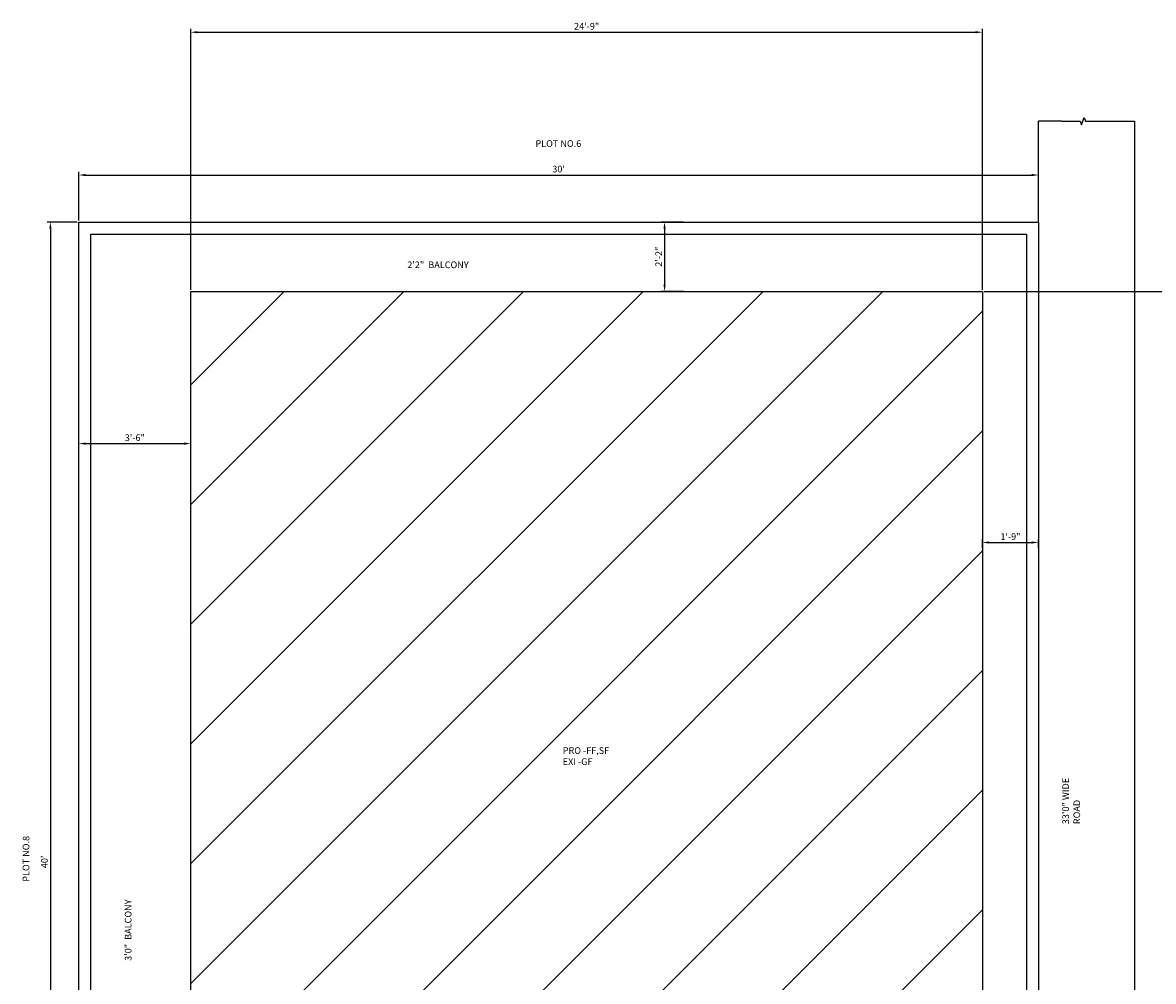
# Model space of a CAD drawing. Units: inches. Extents: x 2020 to 7901, y 1581 to 3943.
# Tile 13 of 17: x 3508 to 3932, y 1955 to 2315. Entities that reach past the tile are written whole.
import ezdxf

# ---------------------------------------------------------------- set-up
doc = ezdxf.new("R2010")
doc.units = ezdxf.units.IN
for name, color, linetype, lineweight in [('A-ANNO-DIMS', 2, 'Continuous', 18), ('A-ANNO-TEXT', 7, 'Continuous', 18), ('A-AREA-IDEN', 3, 'Continuous', 18), ('C-PROP', 6, 'Continuous', 25), ('C-PROP-PATT', 8, 'Continuous', 13)]:
    doc.layers.add(name, color=color, linetype=linetype, lineweight=lineweight)
doc.styles.get("Standard").update_dxf_attribs({"font": 'arial.ttf'})
doc.dimstyles.new('ISO-25', dxfattribs={"dimtxt": 2.5, "dimasz": 2.5, "dimexe": 1.25, "dimexo": 0.625, "dimtad": 1, "dimdec": 1, "dimlunit": 3, "dimtxsty": 'Standard', "dimcen": 2.5, "dimadec": 0, "dimazin": 0, "dimtfac": 1, "dimtdec": 1, "dimtmove": 0, "dimatfit": 3, "dimfxl": 1, "dimarcsym": 0})

# ---------------------------------------------------------------- blocks, each defined once
blk = doc.blocks.new('*D12')
at = {"layer": 'A-ANNO-DIMS', "color": 0, "lineweight": -2, "transparency": 16777216}
for p, q in [((3528.93, 2150.84), (3528.93, 2158.2)), ((3531.43, 2156.95), (3568.43, 2156.95)), ((3570.93, 2150.84), (3570.93, 2158.2))]:
    blk.add_line(p, q, dxfattribs=at)
at = {"layer": 'A-ANNO-DIMS', "color": 0, "transparency": 16777216}
for points in [[(3531.43, 2157.36), (3531.43, 2156.53), (3528.93, 2156.95)], [(3568.43, 2157.36), (3568.43, 2156.53), (3570.93, 2156.95)]]:
    blk.add_solid(points, dxfattribs=at)
at = {"layer": 'DEFPOINTS', "color": 0, "transparency": 16777216}
for p in [(3570.93, 2156.95), (3528.93, 2150.22), (3570.93, 2150.22)]:
    blk.add_point(p, dxfattribs=at)
at = {"layer": 'A-ANNO-DIMS', "color": 0, "transparency": 16777216, "insert": (3549.93, 2158.85), "char_height": 2.5, "attachment_point": 5}
blk.add_mtext('3\'-6"', dxfattribs=at)
blk = doc.blocks.new('*D13')
at = {"layer": 'A-ANNO-DIMS', "color": 0, "lineweight": -2, "transparency": 16777216}
for p, q in [((3755.81, 2240.06), (3747.42, 2240.06)), ((3748.67, 2237.56), (3748.67, 2216.56)), ((3755.81, 2214.06), (3747.42, 2214.06))]:
    blk.add_line(p, q, dxfattribs=at)
at = {"layer": 'A-ANNO-DIMS', "color": 0, "transparency": 16777216}
for points in [[(3748.25, 2237.56), (3749.09, 2237.56), (3748.67, 2240.06)], [(3748.25, 2216.56), (3749.09, 2216.56), (3748.67, 2214.06)]]:
    blk.add_solid(points, dxfattribs=at)
at = {"layer": 'DEFPOINTS', "color": 0, "transparency": 16777216}
for p in [(3756.43, 2240.06), (3748.67, 2214.06), (3756.43, 2214.06)]:
    blk.add_point(p, dxfattribs=at)
at = {"layer": 'A-ANNO-DIMS', "color": 0, "transparency": 16777216, "insert": (3746.79, 2227.06), "char_height": 2.5, "attachment_point": 5, "rotation": 90}
blk.add_mtext('2\'-2"', dxfattribs=at)
blk = doc.blocks.new('*D14')
at = {"layer": 'A-ANNO-DIMS', "color": 0, "lineweight": -2, "transparency": 16777216}
for p, q in [((3867.93, 2117.7), (3867.93, 2121.1)), ((3870.43, 2119.85), (3886.43, 2119.85)), ((3888.93, 2117.7), (3888.93, 2121.1))]:
    blk.add_line(p, q, dxfattribs=at)
at = {"layer": 'A-ANNO-DIMS', "color": 0, "transparency": 16777216}
for points in [[(3870.43, 2120.27), (3870.43, 2119.44), (3867.93, 2119.85)], [(3886.43, 2120.27), (3886.43, 2119.44), (3888.93, 2119.85)]]:
    blk.add_solid(points, dxfattribs=at)
at = {"layer": 'DEFPOINTS', "color": 0, "transparency": 16777216}
for p in [(3867.93, 2117.07), (3888.93, 2119.85), (3888.93, 2117.07)]:
    blk.add_point(p, dxfattribs=at)
at = {"layer": 'A-ANNO-DIMS', "color": 0, "transparency": 16777216, "insert": (3878.43, 2121.75), "char_height": 2.5, "attachment_point": 5}
blk.add_mtext('1\'-9"', dxfattribs=at)
blk = doc.blocks.new('*D15')
at = {"layer": 'A-ANNO-DIMS', "color": 0, "lineweight": -2, "transparency": 16777216}
for p, q in [((3528.93, 2240.68), (3528.93, 2258.94)), ((3531.43, 2257.69), (3886.43, 2257.69)), ((3888.93, 2240.68), (3888.93, 2258.94))]:
    blk.add_line(p, q, dxfattribs=at)
at = {"layer": 'A-ANNO-DIMS', "color": 0, "transparency": 16777216}
for points in [[(3531.43, 2258.1), (3531.43, 2257.27), (3528.93, 2257.69)], [(3886.43, 2258.1), (3886.43, 2257.27), (3888.93, 2257.69)]]:
    blk.add_solid(points, dxfattribs=at)
at = {"layer": 'DEFPOINTS', "color": 0, "transparency": 16777216}
for p in [(3888.93, 2257.69), (3528.93, 2240.06), (3888.93, 2240.06)]:
    blk.add_point(p, dxfattribs=at)
at = {"layer": 'A-ANNO-DIMS', "color": 0, "transparency": 16777216, "insert": (3708.93, 2259.59), "char_height": 2.5, "attachment_point": 5}
blk.add_mtext("30'", dxfattribs=at)
blk = doc.blocks.new('*D16')
at = {"layer": 'A-ANNO-DIMS', "color": 0, "lineweight": -2, "transparency": 16777216}
for p, q in [((3528.3, 2240.06), (3517, 2240.06)), ((3518.25, 2237.56), (3518.25, 1762.56)), ((3528.3, 1760.06), (3517, 1760.06))]:
    blk.add_line(p, q, dxfattribs=at)
at = {"layer": 'A-ANNO-DIMS', "color": 0, "transparency": 16777216}
for points in [[(3517.83, 2237.56), (3518.67, 2237.56), (3518.25, 2240.06)], [(3517.83, 1762.56), (3518.67, 1762.56), (3518.25, 1760.06)]]:
    blk.add_solid(points, dxfattribs=at)
at = {"layer": 'DEFPOINTS', "color": 0, "transparency": 16777216}
for p in [(3528.93, 2240.06), (3518.25, 1760.06), (3528.93, 1760.06)]:
    blk.add_point(p, dxfattribs=at)
at = {"layer": 'A-ANNO-DIMS', "color": 0, "transparency": 16777216, "insert": (3516.35, 2000.06), "char_height": 2.5, "attachment_point": 5, "rotation": 90}
blk.add_mtext("40'", dxfattribs=at)
blk = doc.blocks.new('*D60')
at = {"layer": 'A-ANNO-DIMS', "color": 0, "lineweight": -2, "transparency": 16777216}
for p, q in [((3570.93, 2214.68), (3570.93, 2312.51)), ((3867.93, 2214.68), (3867.93, 2312.51)), ((3573.43, 2311.26), (3865.43, 2311.26))]:
    blk.add_line(p, q, dxfattribs=at)
at = {"layer": 'A-ANNO-DIMS', "color": 0, "transparency": 16777216}
for points in [[(3573.43, 2311.67), (3573.43, 2310.84), (3570.93, 2311.26)], [(3865.43, 2311.67), (3865.43, 2310.84), (3867.93, 2311.26)]]:
    blk.add_solid(points, dxfattribs=at)
at = {"layer": 'DEFPOINTS', "color": 0, "transparency": 16777216}
for p in [(3867.93, 2311.26), (3570.93, 2214.06), (3867.93, 2214.06)]:
    blk.add_point(p, dxfattribs=at)
at = {"layer": 'A-ANNO-DIMS', "color": 0, "transparency": 16777216, "insert": (3719.43, 2313.16), "char_height": 2.5, "attachment_point": 5}
blk.add_mtext('24\'-9"', dxfattribs=at)
blk = doc.blocks.new('*D61')
at = {"layer": 'A-ANNO-DIMS', "color": 0, "lineweight": -2, "transparency": 16777216}
for p, q in [((3868.55, 2214.06), (3980.6, 2214.06)), ((3979.35, 2211.56), (3979.35, 1834.56)), ((3868.55, 1832.06), (3980.6, 1832.06))]:
    blk.add_line(p, q, dxfattribs=at)
at = {"layer": 'A-ANNO-DIMS', "color": 0, "transparency": 16777216}
for points in [[(3978.93, 2211.56), (3979.77, 2211.56), (3979.35, 2214.06)], [(3978.93, 1834.56), (3979.77, 1834.56), (3979.35, 1832.06)]]:
    blk.add_solid(points, dxfattribs=at)
at = {"layer": 'DEFPOINTS', "color": 0, "transparency": 16777216}
for p in [(3867.93, 2214.06), (3867.93, 1832.06), (3979.35, 1832.06)]:
    blk.add_point(p, dxfattribs=at)
at = {"layer": 'A-ANNO-DIMS', "color": 0, "transparency": 16777216, "insert": (3977.45, 2023.06), "char_height": 2.5, "attachment_point": 5, "rotation": 90}
blk.add_mtext('31\'-10"', dxfattribs=at)

msp = doc.modelspace()

# ---------------------------------------------------------------- hatches: boundary and pattern name
at = {"layer": 'C-PROP-PATT'}
h = msp.add_hatch(dxfattribs=at)
h.set_pattern_fill('ANSI31', color=256, scale=10)
h.paths.add_polyline_path([(3867.93, 2214.06), (3570.93, 2214.06), (3570.93, 1832.06), (3867.93, 1832.06)])
h.paths.add_polyline_path([(3709.57, 2034.94), (3730.23, 2034.94), (3730.23, 2044.3), (3709.57, 2044.3)], flags=24)

# ---------------------------------------------------------------- linework, layer by layer
at = {"layer": 'C-PROP'}
for p, q in [((3888.93, 2240.06), (3888.93, 2277.91)), ((3897.59, 2277.84), (3888.93, 2277.84)), ((3906.53, 2277.91), (3912.24, 2277.91)), ((3913.49, 2277.92), (3924.93, 2277.91)), ((3924.93, 2277.91), (3924.93, 1759.48)), ((3528.93, 2240.06), (3888.93, 2240.06)), ((3528.93, 1760.06), (3528.93, 2240.06)), ((3888.93, 2240.06), (3888.93, 1760.06)), ((3533.43, 2235.56), (3884.43, 2235.56)), ((3533.43, 1764.56), (3533.43, 2235.56)), ((3884.43, 2235.56), (3884.43, 1764.56)), ((3570.93, 2214.06), (3867.93, 2214.06)), ((3570.93, 1832.06), (3570.93, 2214.06)), ((3867.93, 2214.06), (3867.93, 1832.06))]:
    msp.add_line(p, q, dxfattribs=at)
for points in [[(3897.59, 2277.84), (3904.54, 2277.87), (3905.04, 2276.5), (3906.03, 2279.26), (3906.54, 2277.88)], [(3912.24, 2277.91), (3913.49, 2277.92)]]:
    msp.add_lwpolyline(points, dxfattribs=at)

# ---------------------------------------------------------------- texts
at = {"layer": 'A-ANNO-TEXT', "char_height": 2.5, "attachment_point": 1}
for s, width, insert in [('2\'2"  BALCONY', 89.6602, (3652.15, 2225.26)), ('PRO -FF,SF\\PEXI -GF', 140.9887, (3710.47, 2043.06))]:
    msp.add_mtext_dynamic_manual_height_columns(s, width=width, gutter_width=12.5, heights=[0], dxfattribs=dict(at, insert=insert))
at = {"layer": 'A-ANNO-TEXT', "char_height": 2.5, "attachment_point": 1, "rotation": 90}
for s, width, insert in [('33\'0" WIDE ROAD', 21.07, (3897.9, 2014.2)), ('3\'0"  BALCONY', 23.8186, (3546.18, 1962.92))]:
    msp.add_mtext_dynamic_manual_height_columns(s, width=width, gutter_width=12.5, heights=[0], dxfattribs=dict(at, insert=insert))
at = {"layer": 'A-AREA-IDEN', "insert": (3700.23, 2270.74), "char_height": 2.5, "attachment_point": 1}
msp.add_mtext_dynamic_manual_height_columns('PLOT NO.6', width=40.3752, gutter_width=12.5, heights=[0], dxfattribs=at)
at = {"layer": 'A-AREA-IDEN', "insert": (3507.88, 1992.6), "char_height": 2.5, "attachment_point": 1, "rotation": 90}
msp.add_mtext_dynamic_manual_height_columns('PLOT NO.8', width=19.8948, gutter_width=12.5, heights=[0], dxfattribs=at)

# ---------------------------------------------------------------- dimensions: what is measured, and where the dimension line sits
at = {"layer": 'A-ANNO-DIMS'}
for base, p1, p2, override, picture, middle in [((3867.93, 2311.26), (3570.93, 2214.06), (3867.93, 2214.06), {"dimdec": 1, "dimlfac": 1, "dimrnd": 0, "dimzin": 1, "dimdsep": 46, "dimlunit": 4, "dimfrac": 2}, '*D60', (3719.43, 2313.16)), ((3888.93, 2257.69), (3528.93, 2240.06), (3888.93, 2240.06), {"dimclrd": 0, "dimclre": 0, "dimclrt": 0}, '*D15', (3708.93, 2259.59)), ((3570.93, 2156.95), (3528.93, 2150.22), (3570.93, 2150.22), {"dimclrd": 0, "dimclre": 0, "dimclrt": 0}, '*D12', (3549.93, 2158.85)), ((3888.93, 2119.85), (3867.93, 2117.07), (3888.93, 2117.07), {"dimclrd": 0, "dimclre": 0, "dimclrt": 0}, '*D14', (3878.43, 2121.75))]:
    dim = msp.add_linear_dim(base=base, p1=p1, p2=p2, dimstyle='ISO-25', override=override, dxfattribs=at)
    dim.commit()
    dim.dimension.update_dxf_attribs({"geometry": picture, "text_midpoint": middle})
for base, p1, p2, override, picture, middle in [((3518.25, 1760.06), (3528.93, 2240.06), (3528.93, 1760.06), {"dimclrd": 0, "dimclre": 0, "dimclrt": 0}, '*D16', (3516.35, 2000.06)), ((3748.67, 2214.06), (3756.43, 2240.06), (3756.43, 2214.06), {"dimclrd": 0, "dimclre": 0, "dimclrt": 0}, '*D13', (3746.79, 2227.06)), ((3979.35, 1832.06), (3867.93, 2214.06), (3867.93, 1832.06), {"dimdec": 1, "dimlfac": 1, "dimrnd": 0, "dimzin": 1, "dimdsep": 46, "dimlunit": 4, "dimfrac": 2}, '*D61', (3977.45, 2023.06))]:
    dim = msp.add_linear_dim(base=base, p1=p1, p2=p2, angle=90, dimstyle='ISO-25', override=override, dxfattribs=at)
    dim.commit()
    dim.dimension.update_dxf_attribs({"geometry": picture, "text_midpoint": middle})

doc.saveas('drawing.dxf')
